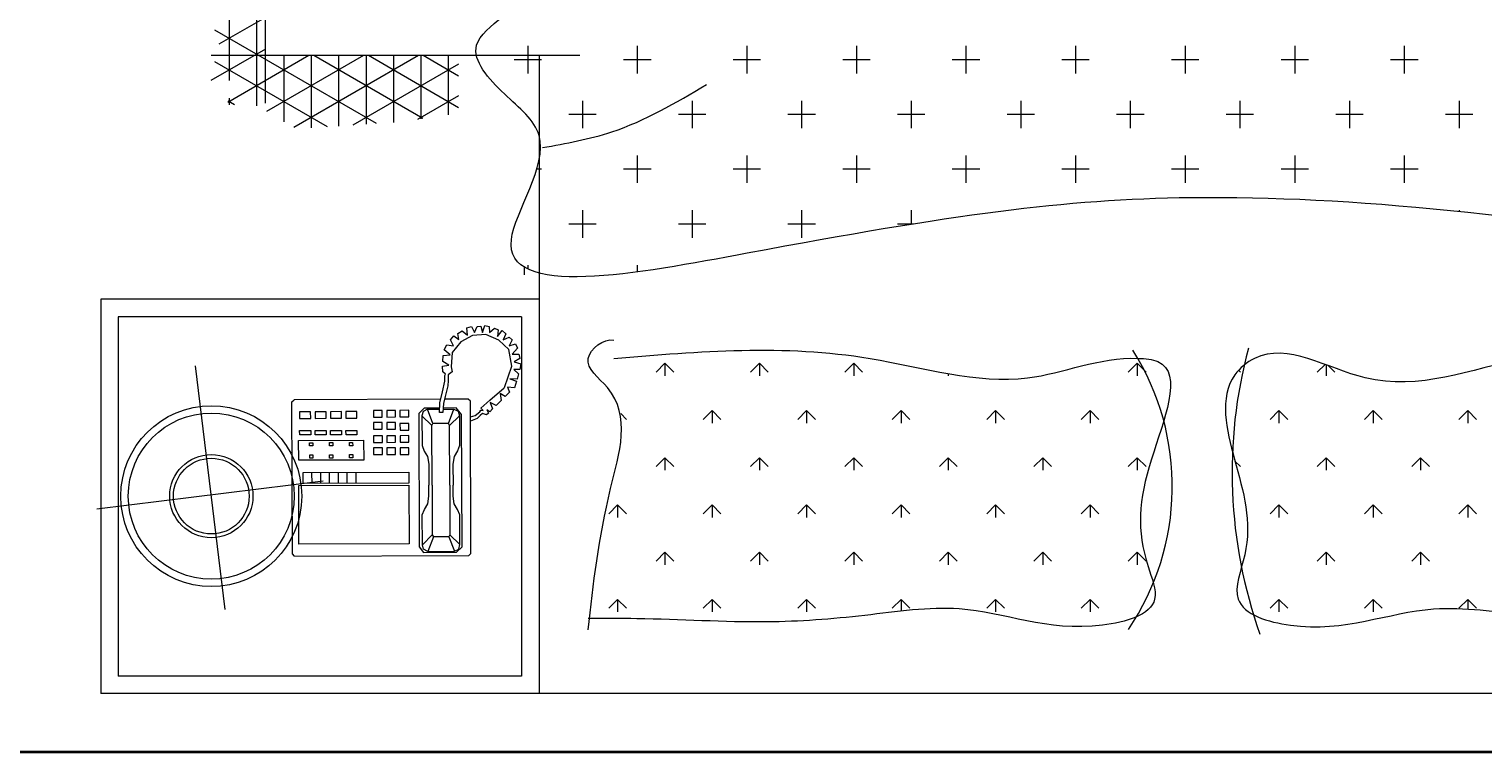
# Model space of a CAD drawing. Units: inches. Extents: x 3731 to 4318, y 1310 to 2388.
# Tile 42 of 57: x 4124 to 4192, y 1943 to 1977. Entities that reach past the tile are written whole.
import ezdxf

# ---------------------------------------------------------------- set-up
doc = ezdxf.new("R2010")
doc.units = ezdxf.units.IN
for name, color, linetype, lineweight in [('A-ANNO-DIMS', 2, 'Continuous', 18), ('A-FURN', 8, 'Continuous', 13), ('A-WALL', 7, 'Continuous', 35)]:
    doc.layers.add(name, color=color, linetype=linetype, lineweight=lineweight)
doc.styles.get("Standard").update_dxf_attribs({"font": 'arial.ttf'})
doc.dimstyles.get("Standard").update_dxf_attribs({"dimtxt": 0.18, "dimasz": 0.18, "dimexe": 0.18, "dimexo": 0.0625, "dimgap": 0.09, "dimtad": 0, "dimtih": 1, "dimtoh": 1, "dimdec": 4, "dimzin": 0, "dimdsep": 46, "dimtxsty": 'Standard', "dimcen": 0.09, "dimadec": 0, "dimazin": 0, "dimtfac": 1, "dimtdec": 4, "dimtofl": 0, "dimtmove": 0, "dimatfit": 3, "dimfxl": 1, "dimtolj": 1, "dimtzin": 0, "dimarcsym": 0})

# ---------------------------------------------------------------- blocks, each defined once
blk = doc.blocks.new('A$C200C7901')
for p, q in [((0.5, 2.3334), (2, 2.3334)), ((2, 2.3334), (2.5, 2.3334)), ((2, 1.6055), (2, 2.3334)), ((2.5, 1.8834), (2.5, 2.3334)), ((0.9943, 2.1721), (0.9842, 2.1822)), ((0.9943, 2.1721), (0.9842, 2.1822)), ((1.3176, 2.1721), (1.3075, 2.1822)), ((1.3176, 2.1721), (1.3075, 2.1822)), ((0.9943, 2.0643), (0.9842, 2.0744)), ((0.9943, 2.0643), (0.9842, 2.0744)), ((1.206, 2.0681), (1.1997, 2.0744)), ((1.206, 2.0681), (1.1997, 2.0744)), ((1.2019, 1.9645), (1.1997, 1.9666)), ((1.2019, 1.9645), (1.1997, 1.9666)), ((2, 1.8834), (2.5, 1.8834)), ((2.0129, 1.8445), (2.0129, 1.849)), ((2.0129, 1.8445), (2.0129, 1.849)), ((2.0171, 1.8467), (2.0171, 1.8556)), ((2.0171, 1.8467), (2.0171, 1.8556)), ((1.1379, 1.7195), (1.1379, 1.7508)), ((1.1222, 1.7352), (1.1535, 1.7352)), ((1.9972, 1.7352), (2.0027, 1.7352)), ((1.9972, 1.7352), (2.0027, 1.7352)), ((2, 1.6963), (2, 1.7248)), ((2, 1.6963), (2, 1.7248)), ((2.3121, 1.6596), (2.3121, 0.0201)), ((1.0129, 1.5945), (1.0129, 1.6258)), ((1.0129, 1.5945), (1.0129, 1.6258)), ((1.9533, 1.6055), (2.3741, 1.6055)), ((1.9533, 1.6055), (2.3741, 1.6055))]:
    blk.add_line(p, q)
at = {"linetype": 'ByBlock'}
for p, q in [((2.02, 2.3134), (2.48, 2.3134)), ((2.02, 1.9034), (2.02, 2.3134)), ((2.48, 1.9034), (2.48, 2.3134)), ((1.0482, 2.2259), (1.0482, 2.2402)), ((1.0482, 2.2259), (1.0482, 2.2402)), ((1.1559, 2.2259), (1.1559, 2.2402)), ((1.1559, 2.2259), (1.1559, 2.2402)), ((1.3714, 2.2259), (1.3714, 2.2402)), ((1.3714, 2.2259), (1.3714, 2.2402)), ((1.4792, 2.2259), (1.4792, 2.2402)), ((1.4792, 2.2259), (1.4792, 2.2402)), ((1.587, 2.2259), (1.587, 2.2393)), ((1.587, 2.2259), (1.587, 2.2393)), ((1.6947, 2.2259), (1.6947, 2.2402)), ((1.6947, 2.2259), (1.6947, 2.2402)), ((1.8025, 2.2259), (1.8025, 2.2402)), ((1.8025, 2.2259), (1.8025, 2.2402)), ((1.9103, 2.2259), (1.9103, 2.2402)), ((1.9103, 2.2259), (1.9103, 2.2402)), ((0.9404, 2.2259), (0.9303, 2.236)), ((0.9404, 2.2259), (0.9303, 2.236)), ((0.9404, 2.2259), (0.9404, 2.2369)), ((0.9404, 2.2259), (0.9404, 2.2369)), ((0.9404, 2.2259), (0.9505, 2.236)), ((0.9404, 2.2259), (0.9505, 2.236)), ((1.0482, 2.2259), (1.0381, 2.236)), ((1.0482, 2.2259), (1.0381, 2.236)), ((1.0482, 2.2259), (1.0583, 2.236)), ((1.0482, 2.2259), (1.0583, 2.236)), ((1.1559, 2.2259), (1.1458, 2.236)), ((1.1559, 2.2259), (1.1458, 2.236)), ((1.1559, 2.2259), (1.166, 2.236)), ((1.1559, 2.2259), (1.166, 2.236)), ((1.3714, 2.2259), (1.3613, 2.236)), ((1.3714, 2.2259), (1.3613, 2.236)), ((1.3714, 2.2259), (1.3815, 2.236)), ((1.3714, 2.2259), (1.3815, 2.236)), ((1.4792, 2.2259), (1.4691, 2.236)), ((1.4792, 2.2259), (1.4691, 2.236)), ((1.4792, 2.2259), (1.4893, 2.236)), ((1.4792, 2.2259), (1.4893, 2.236)), ((1.587, 2.2259), (1.5769, 2.236)), ((1.587, 2.2259), (1.5769, 2.236)), ((1.587, 2.2259), (1.5971, 2.236)), ((1.587, 2.2259), (1.5971, 2.236)), ((1.6947, 2.2259), (1.6846, 2.236)), ((1.6947, 2.2259), (1.6846, 2.236)), ((1.6947, 2.2259), (1.7048, 2.236)), ((1.6947, 2.2259), (1.7048, 2.236)), ((1.8025, 2.2259), (1.7924, 2.236)), ((1.8025, 2.2259), (1.7924, 2.236)), ((1.8025, 2.2259), (1.8126, 2.236)), ((1.8025, 2.2259), (1.8126, 2.236)), ((1.9103, 2.2259), (1.9002, 2.236)), ((1.9103, 2.2259), (1.9002, 2.236)), ((1.9103, 2.2259), (1.9204, 2.236)), ((1.9103, 2.2259), (1.9204, 2.236)), ((2.3581, 2.2373), (2.3919, 1.9595)), ((0.9943, 2.172), (0.9943, 2.1863)), ((0.9943, 2.172), (0.9943, 2.1863)), ((0.9943, 2.1721), (1.0044, 2.1822)), ((0.9943, 2.1721), (1.0044, 2.1822)), ((1.102, 2.1721), (1.0919, 2.1822)), ((1.102, 2.1721), (1.0919, 2.1822)), ((1.102, 2.172), (1.102, 2.1863)), ((1.102, 2.172), (1.102, 2.1863)), ((1.102, 2.1721), (1.1121, 2.1822)), ((1.102, 2.1721), (1.1121, 2.1822)), ((1.3176, 2.172), (1.3176, 2.1863)), ((1.3176, 2.172), (1.3176, 2.1863)), ((1.3176, 2.1721), (1.3277, 2.1822)), ((1.3176, 2.1721), (1.3277, 2.1822)), ((1.4253, 2.1721), (1.4152, 2.1822)), ((1.4253, 2.1721), (1.4152, 2.1822)), ((1.4253, 2.172), (1.4253, 2.1863)), ((1.4253, 2.172), (1.4253, 2.1863)), ((1.4253, 2.1721), (1.4354, 2.1822)), ((1.4253, 2.1721), (1.4354, 2.1822)), ((1.5331, 2.1721), (1.523, 2.1822)), ((1.5331, 2.1721), (1.523, 2.1822)), ((1.5331, 2.172), (1.5331, 2.1863)), ((1.5331, 2.172), (1.5331, 2.1863)), ((1.5331, 2.1721), (1.5432, 2.1822)), ((1.5331, 2.1721), (1.5432, 2.1822)), ((1.6409, 2.1721), (1.6308, 2.1822)), ((1.6409, 2.1721), (1.6308, 2.1822)), ((1.6408, 2.172), (1.6408, 2.1863)), ((1.6408, 2.172), (1.6408, 2.1863)), ((1.6409, 2.1721), (1.651, 2.1822)), ((1.6409, 2.1721), (1.651, 2.1822)), ((1.7486, 2.1721), (1.7385, 2.1822)), ((1.7486, 2.1721), (1.7385, 2.1822)), ((1.7486, 2.172), (1.7486, 2.1863)), ((1.7486, 2.172), (1.7486, 2.1863)), ((1.7486, 2.1721), (1.7587, 2.1822)), ((1.7486, 2.1721), (1.7587, 2.1822)), ((1.8564, 2.1721), (1.8463, 2.1822)), ((1.8564, 2.1721), (1.8463, 2.1822)), ((1.8564, 2.172), (1.8564, 2.1863)), ((1.8564, 2.172), (1.8564, 2.1863)), ((1.8564, 2.1721), (1.8665, 2.1822)), ((1.8564, 2.1721), (1.8665, 2.1822)), ((2.0802, 2.176), (2.0777, 2.1734)), ((2.0777, 2.1734), (2.0783, 1.9999)), ((2.2789, 2.1766), (2.0802, 2.176)), ((2.2789, 2.1766), (2.2814, 2.1741)), ((2.2814, 2.1741), (2.282, 2.0006)), ((2.0941, 2.1722), (2.0878, 2.1659)), ((2.0878, 2.1659), (2.0883, 2.015)), ((2.0915, 2.1685), (2.0903, 2.1634)), ((2.0903, 2.1634), (2.1017, 2.1521)), ((2.0903, 2.1634), (2.0904, 2.1295)), ((2.0966, 2.171), (2.0915, 2.1685)), ((2.1318, 2.1724), (2.0941, 2.1722)), ((2.1267, 2.1711), (2.0966, 2.171)), ((2.1029, 2.1547), (2.0966, 2.171)), ((2.1205, 2.1547), (2.1267, 2.1711)), ((2.1331, 2.1636), (2.1218, 2.1522)), ((2.1267, 2.1711), (2.1318, 2.1686)), ((2.1368, 2.1661), (2.1318, 2.1724)), ((2.1318, 2.1686), (2.1331, 2.1636)), ((2.1331, 2.1636), (2.1332, 2.1296)), ((2.1373, 2.014), (2.1368, 2.1661)), ((2.1481, 2.1624), (2.2739, 2.1628)), ((2.1484, 2.0957), (2.1481, 2.1624)), ((2.2739, 2.1628), (2.2741, 2.0961)), ((2.1017, 2.1521), (2.1029, 2.1547)), ((2.1019, 2.0956), (2.1017, 2.1521)), ((2.1029, 2.1547), (2.1205, 2.1547)), ((2.1218, 2.1522), (2.1205, 2.1547)), ((2.122, 2.0956), (2.1218, 2.1522)), ((0.9404, 2.1182), (0.9303, 2.1283)), ((0.9404, 2.1182), (0.9303, 2.1283)), ((0.9404, 2.1182), (0.9404, 2.1325)), ((0.9404, 2.1182), (0.9404, 2.1325)), ((0.9404, 2.1182), (0.9505, 2.1283)), ((0.9404, 2.1182), (0.9505, 2.1283)), ((1.0482, 2.1182), (1.0381, 2.1283)), ((1.0482, 2.1182), (1.0381, 2.1283)), ((1.0482, 2.1182), (1.0482, 2.1325)), ((1.0482, 2.1182), (1.0482, 2.1325)), ((1.0482, 2.1182), (1.0583, 2.1283)), ((1.0482, 2.1182), (1.0583, 2.1283)), ((1.1559, 2.1182), (1.1458, 2.1283)), ((1.1559, 2.1182), (1.1458, 2.1283)), ((1.1559, 2.1182), (1.1559, 2.1325)), ((1.1559, 2.1182), (1.1559, 2.1325)), ((1.1559, 2.1182), (1.166, 2.1283)), ((1.1559, 2.1182), (1.166, 2.1283)), ((1.3714, 2.1182), (1.3613, 2.1283)), ((1.3714, 2.1182), (1.3613, 2.1283)), ((1.3714, 2.1182), (1.3714, 2.1325)), ((1.3714, 2.1182), (1.3714, 2.1325)), ((1.3714, 2.1182), (1.3815, 2.1283)), ((1.3714, 2.1182), (1.3815, 2.1283)), ((1.4792, 2.1182), (1.4691, 2.1283)), ((1.4792, 2.1182), (1.4691, 2.1283)), ((1.4792, 2.1182), (1.4792, 2.1325)), ((1.4792, 2.1182), (1.4792, 2.1325)), ((1.4792, 2.1182), (1.4893, 2.1283)), ((1.4792, 2.1182), (1.4893, 2.1283)), ((1.587, 2.1182), (1.5769, 2.1283)), ((1.587, 2.1182), (1.5769, 2.1283)), ((1.587, 2.1182), (1.587, 2.1325)), ((1.587, 2.1182), (1.587, 2.1325)), ((1.587, 2.1182), (1.5971, 2.1283)), ((1.587, 2.1182), (1.5971, 2.1283)), ((1.6947, 2.1182), (1.6846, 2.1283)), ((1.6947, 2.1182), (1.6846, 2.1283)), ((1.6947, 2.1182), (1.6947, 2.1325)), ((1.6947, 2.1182), (1.6947, 2.1325)), ((1.6947, 2.1182), (1.7048, 2.1283)), ((1.6947, 2.1182), (1.7048, 2.1283)), ((1.8025, 2.1182), (1.7924, 2.1283)), ((1.8025, 2.1182), (1.7924, 2.1283)), ((1.8025, 2.1182), (1.8025, 2.1325)), ((1.8025, 2.1182), (1.8025, 2.1325)), ((1.8025, 2.1182), (1.8126, 2.1283)), ((1.8025, 2.1182), (1.8126, 2.1283)), ((1.9103, 2.1182), (1.9002, 2.1283)), ((1.9103, 2.1182), (1.9002, 2.1283)), ((1.9103, 2.1182), (1.9103, 2.1325)), ((1.9103, 2.1182), (1.9103, 2.1325)), ((1.9103, 2.1182), (1.9204, 2.1283)), ((1.9103, 2.1182), (1.9204, 2.1283)), ((2.0904, 2.1295), (2.093, 2.1232)), ((2.093, 2.1232), (2.0968, 2.1169)), ((2.1307, 2.1233), (2.1269, 2.117)), ((2.1332, 2.1296), (2.1307, 2.1233)), ((2.0968, 2.1169), (2.098, 2.1081)), ((2.098, 2.1081), (2.0981, 2.0956)), ((2.1269, 2.117), (2.1257, 2.1082)), ((2.1257, 2.1082), (2.1257, 2.0956)), ((2.2464, 2.0911), (2.5044, 2.1228)), ((2.0982, 2.0717), (2.0981, 2.0956)), ((2.1019, 2.0956), (2.1021, 2.0277)), ((2.122, 2.0956), (2.1222, 2.0277)), ((2.1258, 2.0718), (2.1257, 2.0956)), ((2.2741, 2.0961), (2.1484, 2.0957)), ((2.1484, 2.0932), (2.2691, 2.0936)), ((2.1484, 2.0806), (2.1484, 2.0932)), ((2.2087, 2.0934), (2.2088, 2.0808)), ((2.2188, 2.0934), (2.2188, 2.0809)), ((2.2288, 2.0935), (2.2289, 2.0809)), ((2.2389, 2.0935), (2.239, 2.0809)), ((2.249, 2.0935), (2.249, 2.081)), ((2.259, 2.0936), (2.2591, 2.081)), ((2.2691, 2.0936), (2.2691, 2.081)), ((0.9943, 2.0643), (0.9943, 2.0786)), ((0.9943, 2.0643), (0.9943, 2.0786)), ((0.9943, 2.0643), (1.0044, 2.0744)), ((0.9943, 2.0643), (1.0044, 2.0744)), ((1.102, 2.0643), (1.0919, 2.0744)), ((1.102, 2.0643), (1.0919, 2.0744)), ((1.102, 2.0643), (1.102, 2.0786)), ((1.102, 2.0643), (1.102, 2.0786)), ((1.102, 2.0643), (1.1121, 2.0744)), ((1.102, 2.0643), (1.1121, 2.0744)), ((1.3176, 2.0643), (1.3075, 2.0744)), ((1.3176, 2.0643), (1.3075, 2.0744)), ((1.3176, 2.0643), (1.3176, 2.0786)), ((1.3176, 2.0643), (1.3176, 2.0786)), ((1.3176, 2.0643), (1.3277, 2.0744)), ((1.3176, 2.0643), (1.3277, 2.0744)), ((1.4253, 2.0643), (1.4152, 2.0744)), ((1.4253, 2.0643), (1.4152, 2.0744)), ((1.4253, 2.0643), (1.4253, 2.0786)), ((1.4253, 2.0643), (1.4253, 2.0786)), ((1.4253, 2.0643), (1.4354, 2.0744)), ((1.4253, 2.0643), (1.4354, 2.0744)), ((1.5331, 2.0643), (1.523, 2.0744)), ((1.5331, 2.0643), (1.523, 2.0744)), ((1.5331, 2.0643), (1.5331, 2.0786)), ((1.5331, 2.0643), (1.5331, 2.0786)), ((1.5331, 2.0643), (1.5432, 2.0744)), ((1.5331, 2.0643), (1.5432, 2.0744)), ((1.6409, 2.0643), (1.6308, 2.0744)), ((1.6409, 2.0643), (1.6308, 2.0744)), ((1.6408, 2.0643), (1.6408, 2.0786)), ((1.6408, 2.0643), (1.6408, 2.0786)), ((1.6409, 2.0643), (1.651, 2.0744)), ((1.6409, 2.0643), (1.651, 2.0744)), ((1.7486, 2.0643), (1.7385, 2.0744)), ((1.7486, 2.0643), (1.7385, 2.0744)), ((1.7486, 2.0643), (1.7486, 2.0786)), ((1.7486, 2.0643), (1.7486, 2.0786)), ((1.7486, 2.0643), (1.7587, 2.0744)), ((1.7486, 2.0643), (1.7587, 2.0744)), ((1.8564, 2.0643), (1.8463, 2.0744)), ((1.8564, 2.0643), (1.8463, 2.0744)), ((1.8564, 2.0643), (1.8564, 2.0786)), ((1.8564, 2.0643), (1.8564, 2.0786)), ((1.8564, 2.0643), (1.8665, 2.0744)), ((1.8564, 2.0643), (1.8665, 2.0744)), ((2.2691, 2.081), (2.1484, 2.0806)), ((2.0932, 2.0566), (2.0969, 2.0629)), ((2.0969, 2.0629), (2.0982, 2.0717)), ((2.1271, 2.063), (2.1258, 2.0718)), ((2.1309, 2.0567), (2.1271, 2.063)), ((2.1586, 2.0606), (2.1485, 2.0605)), ((2.1485, 2.0605), (2.1485, 2.053)), ((2.1586, 2.053), (2.1586, 2.0606)), ((2.1636, 2.0606), (2.1636, 2.053)), ((2.1736, 2.0606), (2.1636, 2.0606)), ((2.1737, 2.0531), (2.1736, 2.0606)), ((2.1887, 2.0607), (2.1787, 2.0606)), ((2.1787, 2.0606), (2.1787, 2.0531)), ((2.1888, 2.0531), (2.1887, 2.0607)), ((2.2, 2.067), (2.2742, 2.0672)), ((2.2001, 2.0443), (2.2, 2.067)), ((2.2126, 2.0645), (2.2164, 2.0645)), ((2.2126, 2.0607), (2.2126, 2.0645)), ((2.2164, 2.0607), (2.2126, 2.0607)), ((2.2164, 2.0645), (2.2164, 2.0607)), ((2.2352, 2.0646), (2.239, 2.0646)), ((2.2352, 2.0608), (2.2352, 2.0646)), ((2.239, 2.0608), (2.2352, 2.0608)), ((2.239, 2.0646), (2.239, 2.0608)), ((2.2579, 2.0609), (2.2579, 2.0647)), ((2.2579, 2.0647), (2.2616, 2.0647)), ((2.2616, 2.0609), (2.2579, 2.0609)), ((2.2616, 2.0647), (2.2616, 2.0609)), ((2.2742, 2.0672), (2.2743, 2.0446)), ((2.0907, 2.0503), (2.0932, 2.0566)), ((2.0908, 2.0163), (2.0907, 2.0503)), ((2.1334, 2.0504), (2.1309, 2.0567)), ((2.1336, 2.0165), (2.1334, 2.0504)), ((2.1485, 2.053), (2.1586, 2.053)), ((2.1485, 2.0467), (2.1486, 2.0391)), ((2.1586, 2.0467), (2.1485, 2.0467)), ((2.1586, 2.0392), (2.1586, 2.0467)), ((2.1636, 2.053), (2.1737, 2.0531)), ((2.1737, 2.0468), (2.1636, 2.0467)), ((2.1636, 2.0467), (2.1637, 2.0392)), ((2.1737, 2.0392), (2.1737, 2.0468)), ((2.1787, 2.0531), (2.1888, 2.0531)), ((2.1787, 2.0468), (2.1787, 2.0392)), ((2.1888, 2.0468), (2.1787, 2.0468)), ((2.1888, 2.0393), (2.1888, 2.0468)), ((2.2743, 2.0446), (2.2001, 2.0443)), ((2.2126, 2.0507), (2.2164, 2.0507)), ((2.2127, 2.0469), (2.2126, 2.0507)), ((2.2164, 2.0469), (2.2127, 2.0469)), ((2.2164, 2.0507), (2.2164, 2.0469)), ((2.2353, 2.0508), (2.2391, 2.0508)), ((2.2353, 2.047), (2.2353, 2.0508)), ((2.2391, 2.047), (2.2353, 2.047)), ((2.2391, 2.0508), (2.2391, 2.047)), ((2.2579, 2.0508), (2.2617, 2.0508)), ((2.2579, 2.0471), (2.2579, 2.0508)), ((2.2617, 2.0471), (2.2579, 2.0471)), ((2.2617, 2.0508), (2.2617, 2.0471)), ((0.9404, 2.0104), (0.9404, 2.0247)), ((0.9404, 2.0104), (0.9404, 2.0247)), ((1.0482, 2.0104), (1.0482, 2.0247)), ((1.0482, 2.0104), (1.0482, 2.0247)), ((1.1559, 2.0104), (1.1559, 2.0247)), ((1.1559, 2.0104), (1.1559, 2.0247)), ((1.3714, 2.0104), (1.3714, 2.0247)), ((1.3714, 2.0104), (1.3714, 2.0247)), ((1.4792, 2.0104), (1.4792, 2.0247)), ((1.4792, 2.0104), (1.4792, 2.0247)), ((1.587, 2.0104), (1.587, 2.0247)), ((1.587, 2.0104), (1.587, 2.0247)), ((1.6947, 2.0104), (1.6947, 2.0247)), ((1.6947, 2.0104), (1.6947, 2.0247)), ((1.8025, 2.0104), (1.8025, 2.0247)), ((1.8025, 2.0104), (1.8025, 2.0247)), ((2.0908, 2.0163), (2.1021, 2.0277)), ((2.1034, 2.0252), (2.0971, 2.0088)), ((2.1021, 2.0277), (2.1034, 2.0252)), ((2.1034, 2.0252), (2.121, 2.0252)), ((2.1222, 2.0277), (2.121, 2.0252)), ((2.121, 2.0252), (2.1273, 2.0089)), ((2.1336, 2.0165), (2.1222, 2.0277)), ((2.1486, 2.0391), (2.1586, 2.0392)), ((2.1586, 2.0329), (2.1486, 2.0329)), ((2.1486, 2.0329), (2.1486, 2.0253)), ((2.1486, 2.0253), (2.1587, 2.0253)), ((2.1587, 2.0253), (2.1586, 2.0329)), ((2.1637, 2.0392), (2.1737, 2.0392)), ((2.1637, 2.0317), (2.1637, 2.0241)), ((2.1737, 2.0317), (2.1637, 2.0317)), ((2.1637, 2.0241), (2.1738, 2.0241)), ((2.1738, 2.0241), (2.1737, 2.0317)), ((2.1787, 2.0392), (2.1888, 2.0393)), ((2.1788, 2.0317), (2.1788, 2.0242)), ((2.1888, 2.0317), (2.1788, 2.0317)), ((2.1788, 2.0242), (2.1889, 2.0242)), ((2.1889, 2.0242), (2.1888, 2.0317)), ((2.2077, 2.0331), (2.2077, 2.0381)), ((2.2077, 2.0381), (2.2202, 2.0381)), ((2.2203, 2.0331), (2.2077, 2.0331)), ((2.2202, 2.0381), (2.2203, 2.0331)), ((2.2253, 2.0381), (2.2378, 2.0382)), ((2.2253, 2.0331), (2.2253, 2.0381)), ((2.2379, 2.0332), (2.2253, 2.0331)), ((2.2378, 2.0382), (2.2379, 2.0332)), ((2.2429, 2.0332), (2.2429, 2.0382)), ((2.2429, 2.0382), (2.2554, 2.0382)), ((2.2555, 2.0332), (2.2429, 2.0332)), ((2.2554, 2.0382), (2.2555, 2.0332)), ((2.2605, 2.0332), (2.2605, 2.0383)), ((2.2605, 2.0383), (2.273, 2.0383)), ((2.2731, 2.0333), (2.2605, 2.0332)), ((2.273, 2.0383), (2.2731, 2.0333)), ((0.9404, 2.0104), (0.9303, 2.0205)), ((0.9404, 2.0104), (0.9303, 2.0205)), ((0.9404, 2.0104), (0.9505, 2.0205)), ((0.9404, 2.0104), (0.9505, 2.0205)), ((1.0482, 2.0104), (1.0381, 2.0205)), ((1.0482, 2.0104), (1.0381, 2.0205)), ((1.0482, 2.0104), (1.0583, 2.0205)), ((1.0482, 2.0104), (1.0583, 2.0205)), ((1.1559, 2.0104), (1.1458, 2.0205)), ((1.1559, 2.0104), (1.1458, 2.0205)), ((1.1559, 2.0104), (1.166, 2.0205)), ((1.1559, 2.0104), (1.166, 2.0205)), ((1.3714, 2.0104), (1.3613, 2.0205)), ((1.3714, 2.0104), (1.3613, 2.0205)), ((1.3714, 2.0104), (1.3815, 2.0205)), ((1.3714, 2.0104), (1.3815, 2.0205)), ((1.4792, 2.0104), (1.4691, 2.0205)), ((1.4792, 2.0104), (1.4691, 2.0205)), ((1.4792, 2.0104), (1.4893, 2.0205)), ((1.4792, 2.0104), (1.4893, 2.0205)), ((1.587, 2.0104), (1.5769, 2.0205)), ((1.587, 2.0104), (1.5769, 2.0205)), ((1.587, 2.0104), (1.5971, 2.0205)), ((1.587, 2.0104), (1.5971, 2.0205)), ((1.6947, 2.0104), (1.6846, 2.0205)), ((1.6947, 2.0104), (1.6846, 2.0205)), ((1.6947, 2.0104), (1.7048, 2.0205)), ((1.6947, 2.0104), (1.7048, 2.0205)), ((1.8025, 2.0104), (1.7924, 2.0205)), ((1.8025, 2.0104), (1.7924, 2.0205)), ((1.8025, 2.0104), (1.8126, 2.0205)), ((1.8025, 2.0104), (1.8126, 2.0205)), ((1.9068, 2.0139), (1.9002, 2.0205)), ((1.9068, 2.0139), (1.9002, 2.0205)), ((2.053, 2.0084), (2.0563, 2.0119)), ((2.0557, 2.0011), (2.053, 2.0084)), ((2.0663, 2.0077), (2.0561, 1.9986)), ((2.0563, 2.0119), (2.0594, 2.0095)), ((2.0576, 2.0133), (2.0598, 2.0155)), ((2.0594, 2.0095), (2.0576, 2.0133)), ((2.0598, 2.0155), (2.0645, 2.0137)), ((2.0663, 2.0102), (2.0636, 2.0104)), ((2.0636, 2.0104), (2.0663, 2.0077)), ((2.0645, 2.0137), (2.0671, 2.0162)), ((2.0676, 2.012), (2.0663, 2.0102)), ((2.0671, 2.0162), (2.0707, 2.0197)), ((2.0727, 2.016), (2.0676, 2.012)), ((2.0707, 2.0197), (2.0782, 2.0226)), ((2.0782, 2.0175), (2.0727, 2.016)), ((2.0883, 2.015), (2.0946, 2.0075)), ((2.0921, 2.0113), (2.0908, 2.0163)), ((2.0971, 2.0088), (2.0921, 2.0113)), ((2.0946, 2.0075), (2.1093, 2.0076)), ((2.1094, 2.0088), (2.0971, 2.0088)), ((2.109, 2.0025), (2.1097, 2.0126)), ((2.1097, 2.0126), (2.1135, 2.0126)), ((2.1135, 2.0126), (2.1133, 2.0018)), ((2.1273, 2.0089), (2.1134, 2.0088)), ((2.1134, 2.0076), (2.1311, 2.0077)), ((2.1273, 2.0089), (2.1323, 2.0114)), ((2.1311, 2.0077), (2.1373, 2.014)), ((2.1323, 2.0114), (2.1336, 2.0165)), ((2.1587, 2.0178), (2.1486, 2.0178)), ((2.1486, 2.0178), (2.1487, 2.0102)), ((2.1487, 2.0102), (2.1587, 2.0103)), ((2.1587, 2.0103), (2.1587, 2.0178)), ((2.1738, 2.0179), (2.1637, 2.0178)), ((2.1637, 2.0178), (2.1638, 2.0103)), ((2.1638, 2.0103), (2.1738, 2.0103)), ((2.1738, 2.0103), (2.1738, 2.0179)), ((2.1788, 2.0179), (2.1788, 2.0103)), ((2.1889, 2.0179), (2.1788, 2.0179)), ((2.1788, 2.0103), (2.1889, 2.0104)), ((2.1889, 2.0104), (2.1889, 2.0179)), ((2.2203, 2.0193), (2.2077, 2.0192)), ((2.2077, 2.0192), (2.2078, 2.0117)), ((2.2078, 2.0117), (2.2203, 2.0117)), ((2.2203, 2.0117), (2.2203, 2.0193)), ((2.2379, 2.0193), (2.2253, 2.0193)), ((2.2253, 2.0193), (2.2254, 2.0117)), ((2.2254, 2.0117), (2.2379, 2.0118)), ((2.2379, 2.0118), (2.2379, 2.0193)), ((2.2555, 2.0194), (2.2429, 2.0193)), ((2.2429, 2.0193), (2.243, 2.0118)), ((2.243, 2.0118), (2.2555, 2.0118)), ((2.2555, 2.0118), (2.2555, 2.0194)), ((2.2605, 2.0194), (2.2606, 2.0119)), ((2.2731, 2.0194), (2.2605, 2.0194)), ((2.2606, 2.0119), (2.2731, 2.0119)), ((2.2731, 2.0119), (2.2731, 2.0194)), ((2.0338, 1.9895), (2.0386, 1.9946)), ((2.0386, 1.9946), (2.0444, 1.9911)), ((2.0561, 1.9986), (2.0396, 1.9844)), ((2.0431, 1.999), (2.0488, 2.0046)), ((2.0444, 1.9911), (2.0431, 1.999)), ((2.0488, 2.0046), (2.0557, 2.0011)), ((2.0783, 1.9999), (2.0808, 1.9974)), ((2.0808, 1.9974), (2.1079, 1.9975)), ((2.1042, 1.9824), (2.1072, 1.9944)), ((2.1072, 1.9944), (2.109, 2.0025)), ((2.1133, 2.0018), (2.1103, 1.989)), ((2.1123, 1.9975), (2.2795, 1.9981)), ((2.282, 2.0006), (2.2795, 1.9981)), ((2.0234, 1.9686), (2.0251, 1.9745)), ((2.0251, 1.9745), (2.0333, 1.9743)), ((2.0259, 1.977), (2.0281, 1.9847)), ((2.0333, 1.9743), (2.0259, 1.977)), ((2.0281, 1.9847), (2.0358, 1.9839)), ((2.0393, 1.984), (2.031, 1.96)), ((2.0358, 1.9839), (2.0338, 1.9895)), ((2.1035, 1.9763), (2.1042, 1.9824)), ((2.1038, 1.9697), (2.1035, 1.9763)), ((2.1103, 1.989), (2.1073, 1.9771)), ((2.1073, 1.9771), (2.1076, 1.9704)), ((1.0993, 1.9593), (1.0919, 1.9666)), ((1.0993, 1.9593), (1.0919, 1.9666)), ((1.102, 1.9583), (1.102, 1.9708)), ((1.102, 1.9583), (1.102, 1.9708)), ((1.1033, 1.9578), (1.1121, 1.9666)), ((1.1033, 1.9578), (1.1121, 1.9666)), ((1.3176, 1.9565), (1.3075, 1.9666)), ((1.3176, 1.9565), (1.3075, 1.9666)), ((1.3176, 1.9565), (1.3176, 1.9708)), ((1.3176, 1.9565), (1.3176, 1.9708)), ((1.3176, 1.9565), (1.3277, 1.9666)), ((1.3176, 1.9565), (1.3277, 1.9666)), ((1.4253, 1.9703), (1.4253, 1.9708)), ((1.4253, 1.9703), (1.4253, 1.9708)), ((1.5331, 1.9683), (1.5331, 1.9708)), ((1.5331, 1.9683), (1.5331, 1.9708)), ((1.543, 1.9665), (1.5432, 1.9666)), ((1.543, 1.9665), (1.5432, 1.9666)), ((1.6409, 1.9565), (1.6308, 1.9666)), ((1.6409, 1.9565), (1.6308, 1.9666)), ((1.6408, 1.9565), (1.6408, 1.9708)), ((1.6408, 1.9565), (1.6408, 1.9708)), ((1.6409, 1.9565), (1.651, 1.9666)), ((1.6409, 1.9565), (1.651, 1.9666)), ((1.7486, 1.9565), (1.7385, 1.9666)), ((1.7486, 1.9565), (1.7385, 1.9666)), ((1.7486, 1.9565), (1.7486, 1.9708)), ((1.7486, 1.9565), (1.7486, 1.9708)), ((1.7486, 1.9565), (1.7587, 1.9666)), ((1.7486, 1.9565), (1.7587, 1.9666)), ((1.8564, 1.9565), (1.8463, 1.9666)), ((1.8564, 1.9565), (1.8463, 1.9666)), ((1.8564, 1.9565), (1.8564, 1.9708)), ((1.8564, 1.9565), (1.8564, 1.9708)), ((1.8564, 1.9565), (1.8665, 1.9666)), ((1.8564, 1.9565), (1.8665, 1.9666)), ((2.0206, 1.9572), (2.0218, 1.9635)), ((2.0218, 1.9635), (2.0287, 1.9636)), ((2.0287, 1.9636), (2.0234, 1.9686)), ((2.031, 1.96), (2.0346, 1.9409)), ((2.099, 1.9444), (2.1002, 1.9605)), ((2.0992, 1.9663), (2.1038, 1.9697)), ((2.1002, 1.9605), (2.0992, 1.9663)), ((2.1101, 1.96), (2.1028, 1.9587)), ((2.1028, 1.9587), (2.1099, 1.9544)), ((2.1076, 1.9704), (2.1068, 1.9689)), ((2.1068, 1.9689), (2.1096, 1.9661)), ((2.1096, 1.9661), (2.1101, 1.96)), ((2.0285, 1.9549), (2.0206, 1.9572)), ((2.0219, 1.9511), (2.0285, 1.9549)), ((2.0229, 1.946), (2.0219, 1.9511)), ((2.0308, 1.9462), (2.0229, 1.946)), ((2.0247, 1.9394), (2.0308, 1.9462)), ((2.0346, 1.9409), (2.0459, 1.93)), ((2.0894, 1.9322), (2.099, 1.9444)), ((2.1094, 1.9475), (2.1013, 1.9467)), ((2.1013, 1.9467), (2.1084, 1.9412)), ((2.1084, 1.9412), (2.1051, 1.9353)), ((2.1099, 1.9544), (2.1094, 1.9475)), ((2.0268, 1.9343), (2.0247, 1.9394)), ((2.0341, 1.9366), (2.0268, 1.9343)), ((2.0306, 1.9297), (2.0341, 1.9366)), ((2.0339, 1.9267), (2.0306, 1.9297)), ((2.041, 1.9297), (2.0339, 1.9267)), ((2.038, 1.9228), (2.041, 1.9297)), ((2.0474, 1.9259), (2.0421, 1.9193)), ((2.0459, 1.93), (2.0607, 1.9237)), ((2.0467, 1.9183), (2.0474, 1.9259)), ((2.0607, 1.9237), (2.0759, 1.925)), ((2.0759, 1.925), (2.0894, 1.9322)), ((2.0876, 1.9195), (2.0815, 1.9245)), ((2.0815, 1.9245), (2.0823, 1.9161)), ((2.0973, 1.9251), (2.0914, 1.9294)), ((2.0914, 1.9294), (2.0925, 1.9225)), ((2.1011, 1.9297), (2.0973, 1.9251)), ((2.1051, 1.9353), (2.0975, 1.9368)), ((2.0975, 1.9368), (2.1011, 1.9297)), ((2.0421, 1.9193), (2.038, 1.9228)), ((2.0508, 1.9163), (2.0467, 1.9183)), ((2.0566, 1.9214), (2.0508, 1.9163)), ((2.0569, 1.9145), (2.0566, 1.9214)), ((2.0617, 1.9133), (2.0569, 1.9145)), ((2.0645, 1.9214), (2.0617, 1.9133)), ((2.0663, 1.914), (2.0645, 1.9214)), ((2.0706, 1.9146), (2.0663, 1.914)), ((2.0736, 1.9214), (2.0706, 1.9146)), ((2.077, 1.9146), (2.0736, 1.9214)), ((2.0823, 1.9161), (2.077, 1.9146)), ((2.0925, 1.9225), (2.0876, 1.9195)), ((2.02, 1.9034), (2.48, 1.9034)), ((1.8879, 1.8445), (1.8879, 1.8523)), ((1.8879, 1.8445), (1.8879, 1.8523)), ((1.7004, 1.782), (1.7004, 1.8133)), ((1.7004, 1.782), (1.7004, 1.8133)), ((1.8254, 1.782), (1.8254, 1.8133)), ((1.8254, 1.782), (1.8254, 1.8133)), ((1.9504, 1.782), (1.9504, 1.8133)), ((1.9504, 1.782), (1.9504, 1.8133)), ((1.573, 1.7977), (1.591, 1.7977)), ((1.573, 1.7977), (1.591, 1.7977)), ((1.5754, 1.782), (1.5754, 1.7981)), ((1.5754, 1.782), (1.5754, 1.7981)), ((1.6847, 1.7977), (1.716, 1.7977)), ((1.6847, 1.7977), (1.716, 1.7977)), ((1.8097, 1.7977), (1.841, 1.7977)), ((1.8097, 1.7977), (1.841, 1.7977)), ((1.9347, 1.7977), (1.966, 1.7977)), ((1.9347, 1.7977), (1.966, 1.7977)), ((0.9504, 1.782), (0.9504, 1.7836)), ((0.9504, 1.782), (0.9504, 1.7836)), ((1.0129, 1.7195), (1.0129, 1.7508)), ((1.0129, 1.7195), (1.0129, 1.7508)), ((1.1379, 1.7195), (1.1379, 1.7508)), ((1.2629, 1.7195), (1.2629, 1.7508)), ((1.2629, 1.7195), (1.2629, 1.7508)), ((1.3879, 1.7195), (1.3879, 1.7508)), ((1.3879, 1.7195), (1.3879, 1.7508)), ((1.5129, 1.7195), (1.5129, 1.7508)), ((1.5129, 1.7195), (1.5129, 1.7508)), ((1.6379, 1.7195), (1.6379, 1.7508)), ((1.6379, 1.7195), (1.6379, 1.7508)), ((1.7629, 1.7195), (1.7629, 1.7508)), ((1.7629, 1.7195), (1.7629, 1.7508)), ((1.8879, 1.7195), (1.8879, 1.7508)), ((1.8879, 1.7195), (1.8879, 1.7508)), ((0.9972, 1.7352), (1.0285, 1.7352)), ((0.9972, 1.7352), (1.0285, 1.7352)), ((1.1222, 1.7352), (1.1535, 1.7352)), ((1.2472, 1.7352), (1.2785, 1.7352)), ((1.2472, 1.7352), (1.2785, 1.7352)), ((1.3722, 1.7352), (1.4035, 1.7352)), ((1.3722, 1.7352), (1.4035, 1.7352)), ((1.4972, 1.7352), (1.5285, 1.7352)), ((1.4972, 1.7352), (1.5285, 1.7352)), ((1.6222, 1.7352), (1.6535, 1.7352)), ((1.6222, 1.7352), (1.6535, 1.7352)), ((1.7472, 1.7352), (1.7785, 1.7352)), ((1.7472, 1.7352), (1.7785, 1.7352)), ((1.8722, 1.7352), (1.9035, 1.7352)), ((1.8722, 1.7352), (1.9035, 1.7352)), ((0.9504, 1.657), (0.9504, 1.6883)), ((0.9504, 1.657), (0.9504, 1.6883)), ((1.0754, 1.657), (1.0754, 1.6883)), ((1.0754, 1.657), (1.0754, 1.6883)), ((1.2004, 1.657), (1.2004, 1.6883)), ((1.2004, 1.657), (1.2004, 1.6883)), ((1.3254, 1.657), (1.3254, 1.6883)), ((1.3254, 1.657), (1.3254, 1.6883)), ((1.4504, 1.657), (1.4504, 1.6883)), ((1.4504, 1.657), (1.4504, 1.6883)), ((1.5754, 1.657), (1.5754, 1.6883)), ((1.5754, 1.657), (1.5754, 1.6883)), ((1.7004, 1.657), (1.7004, 1.6883)), ((1.7004, 1.657), (1.7004, 1.6883)), ((1.8254, 1.657), (1.8254, 1.6883)), ((1.8254, 1.657), (1.8254, 1.6883)), ((1.9504, 1.657), (1.9504, 1.6883)), ((1.9504, 1.657), (1.9504, 1.6883)), ((2.0919, 1.6152), (2.2125, 1.6848)), ((2.0919, 1.6152), (2.2125, 1.6848)), ((2.0919, 1.6513), (2.1386, 1.6782)), ((2.0919, 1.6513), (2.1386, 1.6782)), ((2.1327, 1.6773), (2.2571, 1.6055)), ((2.1327, 1.6773), (2.2571, 1.6055)), ((2.1349, 1.6055), (2.1349, 1.6777)), ((2.1349, 1.6055), (2.1349, 1.6777)), ((2.1377, 1.6055), (2.2798, 1.6876)), ((2.1377, 1.6055), (2.2798, 1.6876)), ((2.1662, 1.6055), (2.1662, 1.6817)), ((2.1662, 1.6055), (2.1662, 1.6817)), ((2.1854, 1.683), (2.3697, 1.5766)), ((2.1854, 1.683), (2.3697, 1.5766)), ((2.1974, 1.6055), (2.1974, 1.6838)), ((2.1974, 1.6055), (2.1974, 1.6838)), ((2.2287, 1.6055), (2.2287, 1.6859)), ((2.2287, 1.6055), (2.2287, 1.6859)), ((2.2414, 1.6868), (2.3699, 1.6126)), ((2.2414, 1.6868), (2.3699, 1.6126)), ((2.2599, 1.6055), (2.2599, 1.688)), ((2.2599, 1.6055), (2.2599, 1.688)), ((2.2912, 1.6055), (2.2912, 1.6809)), ((2.2912, 1.6055), (2.2912, 1.6809)), ((0.9347, 1.6727), (0.966, 1.6727)), ((0.9347, 1.6727), (0.966, 1.6727)), ((1.0597, 1.6727), (1.091, 1.6727)), ((1.0597, 1.6727), (1.091, 1.6727)), ((1.1847, 1.6727), (1.216, 1.6727)), ((1.1847, 1.6727), (1.216, 1.6727)), ((1.3097, 1.6727), (1.341, 1.6727)), ((1.3097, 1.6727), (1.341, 1.6727)), ((1.4347, 1.6727), (1.466, 1.6727)), ((1.4347, 1.6727), (1.466, 1.6727)), ((1.5597, 1.6727), (1.591, 1.6727)), ((1.5597, 1.6727), (1.591, 1.6727)), ((1.6847, 1.6727), (1.716, 1.6727)), ((1.6847, 1.6727), (1.716, 1.6727)), ((1.8097, 1.6727), (1.841, 1.6727)), ((1.8097, 1.6727), (1.841, 1.6727)), ((1.9347, 1.6727), (1.966, 1.6727)), ((1.9347, 1.6727), (1.966, 1.6727)), ((2.0919, 1.6649), (2.1946, 1.6055)), ((2.0919, 1.6649), (2.1946, 1.6055)), ((2.1037, 1.6055), (2.1037, 1.673)), ((2.1037, 1.6055), (2.1037, 1.673)), ((2.2002, 1.6055), (2.3109, 1.6694)), ((2.2002, 1.6055), (2.3109, 1.6694)), ((2.2627, 1.6055), (2.3551, 1.6589)), ((2.2627, 1.6055), (2.3551, 1.6589)), ((2.3224, 0.0468), (2.3224, 1.6627)), ((2.3224, 0.0468), (2.3224, 1.6627)), ((2.3476, 1.6616), (2.3547, 1.6575)), ((2.3476, 1.6616), (2.3547, 1.6575)), ((2.3537, 1.6539), (2.3537, 1.6616)), ((2.3537, 1.6539), (2.3537, 1.6616)), ((1.1379, 1.5945), (1.1379, 1.6258)), ((1.1379, 1.5945), (1.1379, 1.6258)), ((1.2629, 1.5945), (1.2629, 1.6258)), ((1.2629, 1.5945), (1.2629, 1.6258)), ((1.3879, 1.5945), (1.3879, 1.6258)), ((1.3879, 1.5945), (1.3879, 1.6258)), ((1.5129, 1.5945), (1.5129, 1.6258)), ((1.5129, 1.5945), (1.5129, 1.6258)), ((1.6379, 1.5945), (1.6379, 1.6258)), ((1.6379, 1.5945), (1.6379, 1.6258)), ((1.7629, 1.5945), (1.7629, 1.6258)), ((1.7629, 1.5945), (1.7629, 1.6258)), ((1.8879, 1.5945), (1.8879, 1.6258)), ((1.8879, 1.5945), (1.8879, 1.6258)), ((2.0129, 1.5945), (2.0129, 1.6258)), ((2.0129, 1.5945), (2.0129, 1.6258)), ((2.0919, 1.6288), (2.1321, 1.6055)), ((2.0919, 1.6288), (2.1321, 1.6055)), ((2.3121, 1.598), (2.3745, 1.634)), ((2.3121, 1.598), (2.3745, 1.634)), ((2.3537, 0.0056), (2.3537, 1.634)), ((2.3537, 0.0056), (2.3537, 1.634)), ((0.9972, 1.6102), (1.0285, 1.6102)), ((0.9972, 1.6102), (1.0285, 1.6102)), ((1.1222, 1.6102), (1.1535, 1.6102)), ((1.1222, 1.6102), (1.1535, 1.6102)), ((1.2472, 1.6102), (1.2785, 1.6102)), ((1.2472, 1.6102), (1.2785, 1.6102)), ((1.3722, 1.6102), (1.4035, 1.6102)), ((1.3722, 1.6102), (1.4035, 1.6102)), ((1.4972, 1.6102), (1.5285, 1.6102)), ((1.4972, 1.6102), (1.5285, 1.6102)), ((1.6222, 1.6102), (1.6535, 1.6102)), ((1.6222, 1.6102), (1.6535, 1.6102)), ((1.7472, 1.6102), (1.7785, 1.6102)), ((1.7472, 1.6102), (1.7785, 1.6102)), ((1.8722, 1.6102), (1.9035, 1.6102)), ((1.8722, 1.6102), (1.9035, 1.6102)), ((1.9972, 1.6102), (2.0285, 1.6102)), ((1.9972, 1.6102), (2.0285, 1.6102)), ((2.3121, 1.5619), (2.3654, 1.5926)), ((2.3121, 1.5619), (2.3654, 1.5926))]:
    blk.add_line(p, q, dxfattribs=at)
for radius in [0.1032, 0.0947, 0.0475, 0.0432]:
    blk.add_circle((2.3739, 2.1081), radius, dxfattribs=at)
for centre, radius, start, end in [((0.658, 2.0811), 0.5513, 345.0722, 19.5492), ((1.5685, 2.097), 0.291, 145.8603, 212.2445)]:
    blk.add_arc(centre, radius, start, end)
for points, knots in [([(0.5854, 1.951), (0.6835, 1.9407), (0.8425, 1.9242), (1.0374, 2.0054), (1.1564, 1.9255), (1.2274, 1.9841), (1.2052, 2.0751), (1.1815, 2.152), (1.2176, 2.2368), (1.0992, 2.2731), (1.0008, 2.2255), (0.8698, 2.246), (0.7481, 2.2548), (0.6426, 2.2473), (0.5746, 2.2478), (0.5562, 2.2479)], [0, 0, 0, 0, 292.165466, 473.33038, 601.631673, 630.723769, 727.138505, 836.819956, 887.958136, 954.42438, 1118.989809, 1227.016542, 1338.750986, 1487.447361, 1542.751028, 1542.751028, 1542.751028, 1542.751028]), ([(1.9146, 1.951), (1.8174, 1.9428), (1.6601, 1.9297), (1.4574, 1.9942), (1.3549, 1.9462), (1.2593, 1.9563), (1.314, 2.0834), (1.3193, 2.1569), (1.2853, 2.2393), (1.4031, 2.2724), (1.4987, 2.2256), (1.6304, 2.2459), (1.7519, 2.2548), (1.8574, 2.2473), (1.9254, 2.2478), (1.9438, 2.2479)], [0, 0, 0, 0, 292.165466, 473.33038, 601.631673, 624.236147, 735.870502, 858.452188, 896.317728, 962.783971, 1127.3494, 1235.376134, 1347.110578, 1495.806953, 1551.11062, 1551.11062, 1551.11062, 1551.11062]), ([(1.9438, 2.2608), (1.9381, 2.2086), (1.9282, 2.1195), (1.8897, 2.0022), (1.9591, 1.9538), (1.9264, 1.9278), (1.9146, 1.93)], [0, 0, 0, 0, 163.411291, 278.570782, 318.445997, 354.484131, 354.484131, 354.484131, 354.484131]), ([(0.4485, 1.7835), (0.4321, 1.7496), (0.4062, 1.6964), (0.49, 1.6713), (0.4719, 1.5969), (0.4123, 1.592), (0.4233, 1.5337), (0.4954, 1.5086), (0.4012, 1.4738), (0.3253, 1.4306), (0.4113, 1.3764), (0.3688, 1.3065), (0.5579, 1.2663), (0.741, 1.4533), (1.1127, 1.1109), (1.4811, 1.2478), (1.7885, 1.3492), (2.0357, 1.1637), (2.0748, 1.2974), (2.0876, 1.349), (2.0192, 1.3805), (2.0564, 1.4298), (2.0588, 1.4846), (1.9759, 1.5349), (2.1004, 1.5845), (2.0397, 1.6519), (1.971, 1.7053), (2.1104, 1.8981), (1.5946, 1.7967), (1.2448, 1.7472), (0.8129, 1.7935), (0.4953, 1.8548), (0.4582, 1.7983), (0.4485, 1.7835)], [0, 0, 0, 0, 88.420092, 139.08588, 204.302936, 239.695496, 287.801042, 327.365471, 412.960499, 463.626286, 552.059846, 584.668336, 662.614915, 940.993281, 1309.926334, 1844.022653, 1996.276242, 2316.43048, 2341.441004, 2404.707416, 2449.463774, 2514.680778, 2538.40571, 2613.031547, 2697.13096, 2760.903931, 2822.692699, 2945.47, 3215.060018, 3725.584917, 4361.974444, 4504.671998, 4555.32777, 4555.32777, 4555.32777, 4555.32777])]:
    blk.add_open_spline(points, degree=3, knots=knots)
blk.add_open_spline([(1.996, 1.7104), (1.9692, 1.7057), (1.9025, 1.6938), (1.844, 1.6592), (1.809, 1.6385)], degree=3, knots=[0, 0, 0, 0, 81.132613, 201.738644, 201.738644, 201.738644, 201.738644], dxfattribs=at)
blk.add_open_spline([(1.996, 1.7104), (1.9692, 1.7057), (1.9025, 1.6938), (1.844, 1.6592), (1.809, 1.6385)], degree=3, knots=[0, 0, 0, 0, 81.132613, 201.738644, 201.738644, 201.738644, 201.738644], dxfattribs=at)
blk = doc.blocks.new('*D38')
at = {"layer": 'A-ANNO-DIMS', "color": 0, "lineweight": -2, "transparency": 16777216}
for p, q in [((4103.271, 2262.382), (4318.341, 2262.382)), ((4318.161, 2262.202), (4318.161, 2103.064)), ((4318.161, 1943.562), (4318.161, 2102.7)), ((4234.271, 1943.382), (4318.341, 1943.382))]:
    blk.add_line(p, q, dxfattribs=at)
at = {"layer": 'A-ANNO-DIMS', "color": 0, "transparency": 16777216}
for points in [[(4318.131, 2262.202), (4318.191, 2262.202), (4318.161, 2262.382)], [(4318.131, 1943.562), (4318.191, 1943.562), (4318.161, 1943.382)]]:
    blk.add_solid(points, dxfattribs=at)
at = {"layer": 'Defpoints', "color": 0, "transparency": 16777216}
for p in [(4103.209, 2262.382), (4318.161, 2262.382), (4234.209, 1943.382)]:
    blk.add_point(p, dxfattribs=at)
at = {"layer": 'A-ANNO-DIMS', "color": 0, "transparency": 16777216, "insert": (4318.161, 2102.882), "char_height": 0.18, "attachment_point": 5}
blk.add_mtext('\\A1;319', dxfattribs=at)

msp = doc.modelspace()

# ---------------------------------------------------------------- linework, layer by layer
at = {"layer": 'A-WALL'}
msp.add_line((4108.209, 1943.382), (4234.209, 1943.382), dxfattribs=at)

# ---------------------------------------------------------------- block references
at = {"layer": 'A-FURN', "xscale": 41.1071563136412, "yscale": 41.1071563136412, "zscale": 41.1071563136412, "rotation": 180}
msp.add_blockref('A$C200C7901', (4230.145, 2042.037), dxfattribs=at)

# ---------------------------------------------------------------- dimensions: what is measured, and where the dimension line sits
at = {"layer": 'A-ANNO-DIMS'}
dim = msp.add_linear_dim(base=(4318.161, 2262.382), p1=(4234.209, 1943.382), p2=(4103.209, 2262.382), angle=90, dimstyle='Standard', override={"dimdec": 0, "dimlfac": 1, "dimrnd": 0, "dimzin": 0, "dimdsep": 46, "dimlunit": 2}, dxfattribs=at)
dim.commit()
dim.dimension.update_dxf_attribs({"geometry": '*D38', "text_midpoint": (4318.161, 2102.882)})

doc.saveas('drawing.dxf')
